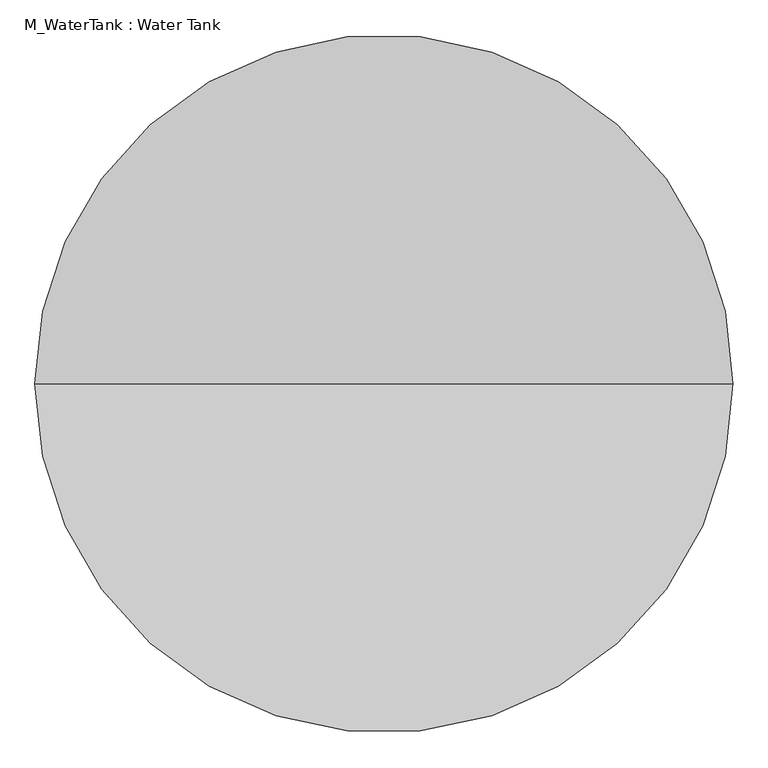
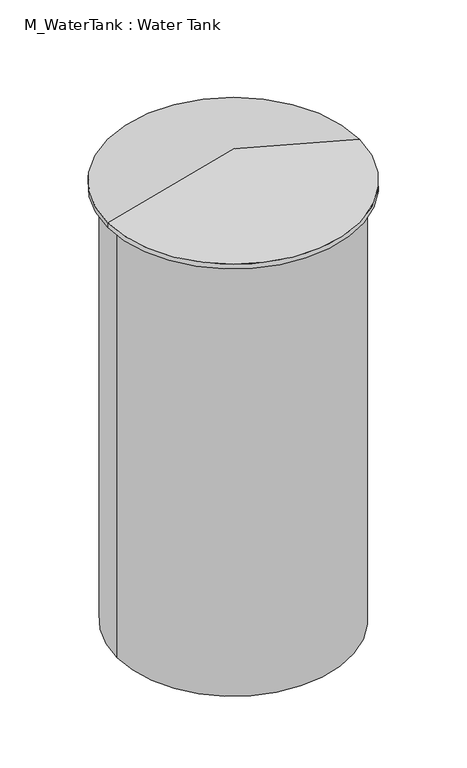
"""IFC4 building model written with IfcOpenShell, lengths in millimetres: proxy geometry, M_WaterTank : Water Tank."""

from ifc_helpers import new_model, si_unit, point, frame, origin, origin_with_axes, origin_2d, place, context, project, spatial, polyline, circle_curve, trimmed, segment, composite_curve, outline, extrude, source, transform, mapped, element, save
from ifc_brep_helpers import plane_surface, cylinder_surface, revolved_surface, advanced_brep


def m_watertank_water_tank_eee2c874(model_context):
    return source(origin(), model_context, "Body", "SolidModel", [
        extrude(outline(composite_curve([segment(trimmed(circle_curve(origin_2d(), 915.0), [point((-915.0, 0.0))], [point((915.0, 0.0))], False, "CARTESIAN"), True, "CONTINUOUS"), segment(trimmed(circle_curve(origin_2d(), 915.0), [point((915.0, 0.0))], [point((-915.0, 0.0))], False, "CARTESIAN"), True, "CONTINUOUS")], self_intersect=False)), origin_with_axes(), (0.0, 0.0, 1.0), 3600.0),
        advanced_brep(
        [(990.0, 0.0, 3639.7302995), (-990.0, 0.0, 3639.7302995), (0.0, 0.0, 3905.0), (990.0, 0.0, 3600.0), (-990.0, 0.0, 3600.0), (0.0, 0.0, 3600.0)],
        [
            (0, 1, circle_curve(frame((0.0, 0.0, 3639.7302995), z_axis=(0.0, 0.0, 1.0), x_axis=(-1.0, 0.0, 0.0)), 990.0)),
            (1, 2),
            (2, 0),
            (1, 0, circle_curve(frame((0.0, 0.0, 3639.7302995), z_axis=(0.0, 0.0, 1.0), x_axis=(-1.0, 0.0, 0.0)), 990.0)),
            (3, 4, circle_curve(frame((0.0, 0.0, 3600.0), z_axis=(0.0, 0.0, 1.0), x_axis=(-1.0, 0.0, 0.0)), 990.0)),
            (4, 1),
            (0, 3),
            (4, 3, circle_curve(frame((0.0, 0.0, 3600.0), z_axis=(0.0, 0.0, 1.0), x_axis=(-1.0, 0.0, 0.0)), 990.0)),
            (5, 4),
            (3, 5),
        ],
        [
            revolved_surface(polyline([(0.0, 0.0, 3905.0), (-990.0, 0.0, 3639.7302995)]), (0.0, 0.0, 3600.0), (0.0, 0.0, -1.0)),
            cylinder_surface(frame((0.0, 0.0, 3600.0), z_axis=(0.0, 0.0, -1.0), x_axis=(-1.0, 0.0, 0.0)), 990.0),
            plane_surface(frame((0.0, 0.0, 3600.0), z_axis=(0.0, 0.0, -1.0), x_axis=(-1.0, 0.0, 0.0))),
        ],
        [
            (0, [[1, 2, 3]]),
            (0, [[4, -3, -2]]),
            (1, [[5, 6, -1, 7]]),
            (1, [[8, -7, -4, -6]]),
            (2, [[9, -5, 10]]),
            (2, [[-10, -8, -9]]),
        ],
    ),
    ])


if __name__ == "__main__":
    model = new_model("IFC4")
    model_context = context("Model", 3, world=origin())
    ifc_project = project(units=[si_unit("LENGTHUNIT", "METRE", prefix="MILLI")], contexts=[model_context])
    site = spatial("IfcSite", under=ifc_project)
    building = spatial("IfcBuilding", under=site)
    placement = place(None, origin())
    m_watertank_water_tank_shape = m_watertank_water_tank_eee2c874(model_context)
    element("IfcBuildingElementProxy", 1, Name="M_WaterTank : Water Tank", ObjectType="M_WaterTank : Water Tank", at=placement, inside=building, context=model_context, shape_type="MappedRepresentation", body=[
        mapped(m_watertank_water_tank_shape, transform((0.0, 0.0, 0.0), x_axis=(1.0, 0.0, 0.0), y_axis=(0.0, 1.0, 0.0), z_axis=(0.0, 0.0, 1.0))),
    ])
    save(model, "model.ifc")

# Revit data of these elements
# Type "M_WaterTank : Water Tank"
#   Width Of Top = 3' - 2.97638"
#   Radius = 3' - 0.02362"
#   Height = 11' - 9.73228"
#   Default Elevation = 0
